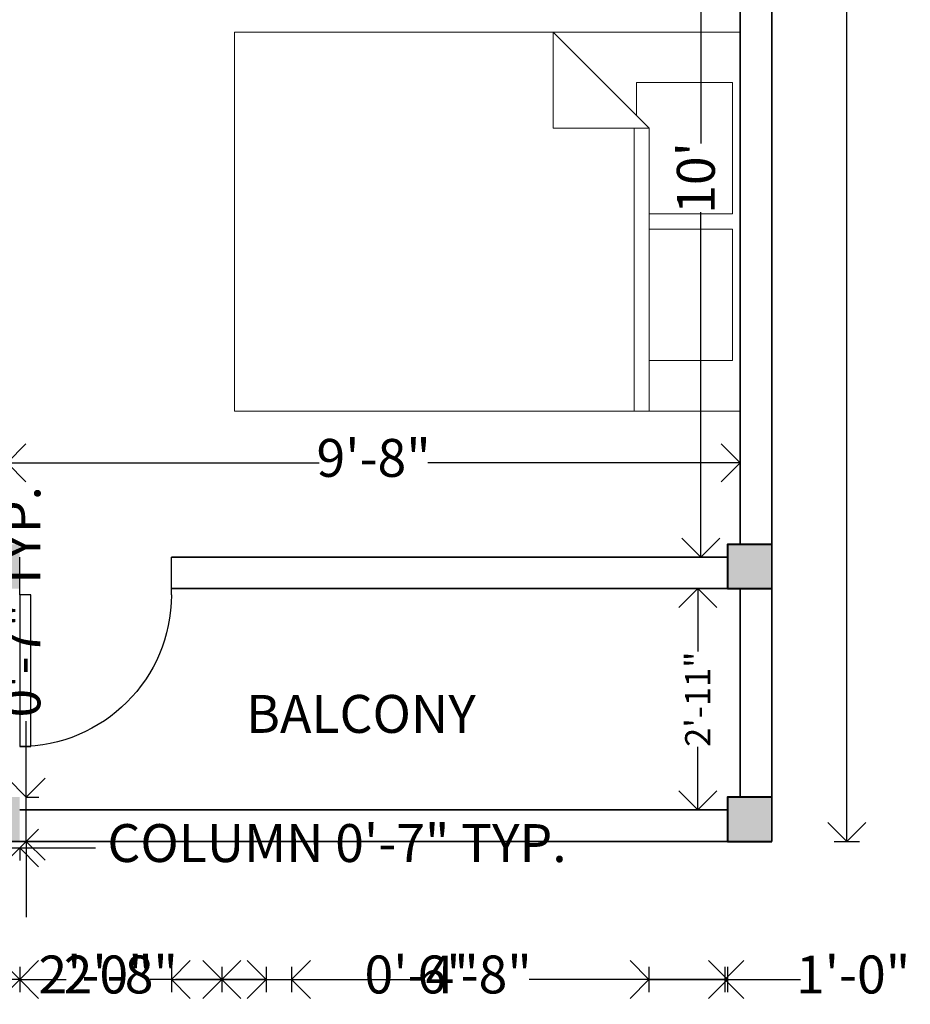
# Model space of a CAD drawing. Units: inches. Extents: x 261 to 714, y 97 to 573.
# Tile 3 of 5: x 541 to 682, y 97 to 253. Entities that reach past the tile are written whole.
import ezdxf

# ---------------------------------------------------------------- set-up
doc = ezdxf.new("R2010")
doc.units = ezdxf.units.IN
for name, color, linetype, lineweight in [('A-ANNO-DIMS', 2, 'Continuous', 18), ('A-AREA-IDEN', 7, 'Continuous', 25), ('A-COLS', 182, 'Continuous', 40), ('A-COLS-PATT', 172, 'Continuous', 13), ('A-DOOR', 182, 'Continuous', 25), ('A-FURN', 8, 'Continuous', 18), ('A-WALL', 182, 'Continuous', 35)]:
    doc.layers.add(name, color=color, linetype=linetype, lineweight=lineweight)
doc.styles.get("Standard").update_dxf_attribs({"font": 'arial.ttf'})
doc.dimstyles.new('ISO-25', dxfattribs={"dimtxt": 6, "dimasz": 6, "dimexe": 2, "dimexo": 2, "dimtad": 0, "dimdec": 1, "dimlunit": 3, "dimtxsty": 'Standard', "dimblk": 'OPEN90', "dimcen": 2.5, "dimclrd": 1, "dimclre": 1, "dimclrt": 1, "dimadec": 0, "dimazin": 0, "dimtfac": 1, "dimtdec": 1, "dimtmove": 0, "dimatfit": 3, "dimfxl": 2, "dimfxlon": 1, "dimarcsym": 0})

# ---------------------------------------------------------------- blocks, each defined once
blk = doc.blocks.new('*U6')
for p, q in [((0, 0), (0, -6)), ((24, 0), (24, -6))]:
    blk.add_line(p, q)
blk.add_lwpolyline([(0, 0), (0, 24), (1.75, 24), (1.75, 0)], close=True)
blk.add_arc((0, 0), 24, 0, 90)
blk = doc.blocks.new('_Open90')
at = {"color": 0, "linetype": 'ByBlock', "lineweight": -2}
for p, q in [((-0.5, 0.5), (0, 0)), ((0, 0), (-1, 0)), ((0, 0), (-0.5, -0.5))]:
    blk.add_line(p, q, dxfattribs=at)
blk = doc.blocks.new('*D21')
at = {"layer": 'A-ANNO-DIMS', "color": 0, "lineweight": -2, "transparency": 16777216}
for p, q in [((646.66, 287.66), (650.66, 287.66)), ((648.66, 281.66), (648.66, 233.09)), ((648.66, 173.66), (648.66, 222.22)), ((646.66, 167.66), (650.66, 167.66))]:
    blk.add_line(p, q, dxfattribs=at)
at = {"layer": 'Defpoints', "color": 0, "transparency": 16777216}
for p in [(643.84, 287.66), (643.84, 167.66), (648.66, 167.66)]:
    blk.add_point(p, dxfattribs=at)
at = {"layer": 'A-ANNO-DIMS', "color": 0, "lineweight": -2, "transparency": 16777216, "xscale": 6, "yscale": 6, "zscale": 6}
for p, rotation in [((648.66, 287.66), 90), ((648.66, 167.66), 270)]:
    blk.add_blockref('_Open90', p, dxfattribs=dict(at, rotation=rotation))
at = {"layer": 'A-ANNO-DIMS', "color": 0, "transparency": 16777216, "insert": (648.66, 227.66), "char_height": 6, "attachment_point": 5, "rotation": 90}
blk.add_mtext("10'", dxfattribs=at)
blk = doc.blocks.new('*D22')
at = {"layer": 'A-ANNO-DIMS', "color": 0, "lineweight": -2, "transparency": 16777216}
for p, q in [((538.9, 184.57), (538.9, 180.57)), ((654.9, 184.57), (654.9, 180.57)), ((544.9, 182.57), (588.3, 182.57)), ((648.9, 182.57), (605.5, 182.57))]:
    blk.add_line(p, q, dxfattribs=at)
at = {"layer": 'Defpoints', "color": 0, "transparency": 16777216}
for p in [(538.9, 189.8), (654.9, 189.8), (654.9, 182.57)]:
    blk.add_point(p, dxfattribs=at)
at = {"layer": 'A-ANNO-DIMS', "color": 0, "lineweight": -2, "transparency": 16777216, "xscale": 6, "yscale": 6, "zscale": 6, "rotation": 180}
blk.add_blockref('_Open90', (538.9, 182.57), dxfattribs=at)
at = {"layer": 'A-ANNO-DIMS', "color": 0, "lineweight": -2, "transparency": 16777216, "xscale": 6, "yscale": 6, "zscale": 6}
blk.add_blockref('_Open90', (654.9, 182.57), dxfattribs=at)
at = {"layer": 'A-ANNO-DIMS', "color": 0, "transparency": 16777216, "insert": (596.9, 182.57), "char_height": 6, "attachment_point": 5}
blk.add_mtext('9\'-8"', dxfattribs=at)
blk = doc.blocks.new('*D24')
at = {"layer": 'A-ANNO-DIMS', "color": 0, "lineweight": -2, "transparency": 16777216}
for p, q in [((650.18, 162.66), (646.18, 162.66)), ((648.18, 156.66), (648.18, 152.69)), ((648.18, 133.66), (648.18, 137.63)), ((650.18, 127.66), (646.18, 127.66))]:
    blk.add_line(p, q, dxfattribs=at)
at = {"layer": 'Defpoints', "color": 0, "transparency": 16777216}
for p in [(662.6, 162.66), (648.18, 127.66), (662.6, 127.66)]:
    blk.add_point(p, dxfattribs=at)
at = {"layer": 'A-ANNO-DIMS', "color": 0, "lineweight": -2, "transparency": 16777216, "xscale": 6, "yscale": 6, "zscale": 6}
for p, rotation in [((648.18, 162.66), 90), ((648.18, 127.66), 270)]:
    blk.add_blockref('_Open90', p, dxfattribs=dict(at, rotation=rotation))
at = {"layer": 'A-ANNO-DIMS', "color": 0, "transparency": 16777216, "insert": (648.18, 145.16), "char_height": 6, "attachment_point": 5, "rotation": 90}
blk.add_mtext('{\\H0.66667x;2\'-11"}', dxfattribs=at)
blk = doc.blocks.new('Bed - Queen')
for p, q in [((0, -80.00003), (0, 0)), ((0, 0), (59.99999, 0)), ((59.99999, 0), (59.99999, -80.00003)), ((7.99999, -1.2), (28.79998, -1.2)), ((7.99999, -14.4), (7.99999, -1.2)), ((28.79998, -1.2), (28.79998, -14.4)), ((31.19999, -1.2), (51.99999, -1.2)), ((31.19999, -14.4), (31.19999, -1.2)), ((51.99999, -1.2), (51.99999, -16.4)), ((0, -14.4), (44.8, -14.4)), ((59.99999, -29.6), (44.8, -14.4)), ((44.8, -14.4), (44.8, -29.6)), ((44.8, -16.8), (0, -16.8)), ((51.99999, -16.4), (46.79936, -16.4)), ((44.8, -29.6), (59.99999, -29.6)), ((59.99999, -80.00003), (0, -80.00003))]:
    blk.add_line(p, q)
blk = doc.blocks.new('*D35')
at = {"layer": 'A-ANNO-DIMS', "color": 0, "lineweight": -2, "transparency": 16777216}
for p, q in [((669.78, 542.66), (673.78, 542.66)), ((671.78, 536.66), (671.78, 338.37)), ((671.78, 128.66), (671.78, 326.94)), ((669.78, 122.66), (673.78, 122.66))]:
    blk.add_line(p, q, dxfattribs=at)
at = {"layer": 'Defpoints', "color": 0, "transparency": 16777216}
for p in [(659.9, 542.66), (659.9, 122.66), (671.78, 122.66)]:
    blk.add_point(p, dxfattribs=at)
at = {"layer": 'A-ANNO-DIMS', "color": 0, "lineweight": -2, "transparency": 16777216, "xscale": 6, "yscale": 6, "zscale": 6}
for p, rotation in [((671.78, 542.66), 90), ((671.78, 122.66), 270)]:
    blk.add_blockref('_Open90', p, dxfattribs=dict(at, rotation=rotation))
at = {"layer": 'A-ANNO-DIMS', "color": 0, "transparency": 16777216, "insert": (671.78, 332.66), "char_height": 6, "attachment_point": 5, "rotation": 90}
blk.add_mtext("35'", dxfattribs=at)
blk = doc.blocks.new('COLUMN-7IN-SIDE-EDGE')
blk.add_lwpolyline([(7, 7), (0, 7), (0, 2), (0, 0), (2, 0), (7, 0)])
blk = doc.blocks.new('*D41')
at = {"layer": 'A-ANNO-DIMS', "color": 1, "lineweight": -2, "transparency": 16777216}
for p, q in [((527.9, 121.61), (521.9, 121.61)), ((533.9, 121.61), (533.9, 119.61)), ((533.9, 121.61), (540.9, 121.61)), ((540.9, 121.61), (540.9, 119.61)), ((546.9, 121.61), (552.9, 121.61))]:
    blk.add_line(p, q, dxfattribs=at)
at = {"layer": 'Defpoints', "color": 0, "transparency": 16777216}
for p in [(533.9, 122.66), (540.9, 122.66), (540.9, 121.61)]:
    blk.add_point(p, dxfattribs=at)
at = {"layer": 'A-ANNO-DIMS', "color": 1, "lineweight": -2, "transparency": 16777216, "xscale": 6, "yscale": 6, "zscale": 6}
blk.add_blockref('_Open90', (533.9, 121.61), dxfattribs=at)
at = {"layer": 'A-ANNO-DIMS', "color": 1, "lineweight": -2, "transparency": 16777216, "xscale": 6, "yscale": 6, "zscale": 6, "rotation": 180}
blk.add_blockref('_Open90', (540.9, 121.61), dxfattribs=at)
at = {"layer": 'A-ANNO-DIMS', "color": 1, "transparency": 16777216, "insert": (591.11, 121.61), "char_height": 6, "attachment_point": 5}
blk.add_mtext('COLUMN 0\'-7" TYP.', dxfattribs=at)
blk = doc.blocks.new('*D42')
at = {"layer": 'A-ANNO-DIMS', "color": 1, "lineweight": -2, "transparency": 16777216}
for p, q in [((541.95, 135.66), (541.95, 141.66)), ((541.95, 129.66), (543.95, 129.66)), ((541.95, 122.66), (541.95, 129.66)), ((541.95, 122.66), (543.95, 122.66)), ((541.95, 116.66), (541.95, 110.66))]:
    blk.add_line(p, q, dxfattribs=at)
at = {"layer": 'Defpoints', "color": 0, "transparency": 16777216}
for p in [(540.9, 129.66), (541.95, 129.66), (540.9, 122.66)]:
    blk.add_point(p, dxfattribs=at)
at = {"layer": 'A-ANNO-DIMS', "color": 1, "lineweight": -2, "transparency": 16777216, "xscale": 6, "yscale": 6, "zscale": 6}
for p, rotation in [((541.95, 129.66), 270), ((541.95, 122.66), 90)]:
    blk.add_blockref('_Open90', p, dxfattribs=dict(at, rotation=rotation))
at = {"layer": 'A-ANNO-DIMS', "color": 1, "transparency": 16777216, "insert": (541.95, 160.57), "char_height": 6, "attachment_point": 5, "rotation": 90}
blk.add_mtext('0\'-7" TYP.', dxfattribs=at)
blk = doc.blocks.new('*D63')
at = {"layer": 'A-ANNO-DIMS', "color": 1, "lineweight": -2, "transparency": 16777216}
for p, q in [((540.9, 102.81), (540.9, 98.81)), ((572.9, 102.81), (572.9, 98.81)), ((546.9, 100.81), (548.25, 100.81)), ((566.9, 100.81), (565.55, 100.81))]:
    blk.add_line(p, q, dxfattribs=at)
at = {"layer": 'Defpoints', "color": 0, "transparency": 16777216}
for p in [(540.9, 287.66), (572.9, 287.66), (572.9, 100.81)]:
    blk.add_point(p, dxfattribs=at)
at = {"layer": 'A-ANNO-DIMS', "color": 1, "lineweight": -2, "transparency": 16777216, "xscale": 6, "yscale": 6, "zscale": 6, "rotation": 180}
blk.add_blockref('_Open90', (540.9, 100.81), dxfattribs=at)
at = {"layer": 'A-ANNO-DIMS', "color": 1, "lineweight": -2, "transparency": 16777216, "xscale": 6, "yscale": 6, "zscale": 6}
blk.add_blockref('_Open90', (572.9, 100.81), dxfattribs=at)
at = {"layer": 'A-ANNO-DIMS', "color": 1, "transparency": 16777216, "insert": (556.9, 100.81), "char_height": 6, "attachment_point": 5}
blk.add_mtext('2\'-8"', dxfattribs=at)
blk = doc.blocks.new('*D64')
at = {"layer": 'A-ANNO-DIMS', "color": 1, "lineweight": -2, "transparency": 16777216}
for p, q in [((572.9, 102.81), (572.9, 98.81)), ((652.88, 102.81), (652.88, 98.81)), ((578.9, 100.81), (604.28, 100.81)), ((646.88, 100.81), (621.51, 100.81))]:
    blk.add_line(p, q, dxfattribs=at)
at = {"layer": 'Defpoints', "color": 0, "transparency": 16777216}
for p in [(572.9, 287.66), (652.88, 287.66), (652.88, 100.81)]:
    blk.add_point(p, dxfattribs=at)
at = {"layer": 'A-ANNO-DIMS', "color": 1, "lineweight": -2, "transparency": 16777216, "xscale": 6, "yscale": 6, "zscale": 6, "rotation": 180}
blk.add_blockref('_Open90', (572.9, 100.81), dxfattribs=at)
at = {"layer": 'A-ANNO-DIMS', "color": 1, "lineweight": -2, "transparency": 16777216, "xscale": 6, "yscale": 6, "zscale": 6}
blk.add_blockref('_Open90', (652.88, 100.81), dxfattribs=at)
at = {"layer": 'A-ANNO-DIMS', "color": 1, "transparency": 16777216, "insert": (612.89, 100.81), "char_height": 6, "attachment_point": 5}
blk.add_mtext('6\'-8"', dxfattribs=at)
blk = doc.blocks.new('*D66')
at = {"layer": 'A-ANNO-DIMS', "color": 1, "lineweight": -2, "transparency": 16777216}
for p, q in [((540.9, 102.81), (540.9, 98.81)), ((564.9, 102.81), (564.9, 98.81)), ((534.9, 100.81), (528.9, 100.81)), ((540.9, 100.81), (544.25, 100.81)), ((564.9, 100.81), (561.55, 100.81)), ((570.9, 100.81), (576.9, 100.81))]:
    blk.add_line(p, q, dxfattribs=at)
at = {"layer": 'Defpoints', "color": 0, "transparency": 16777216}
for p in [(540.9, 162.66), (564.9, 162.66), (564.9, 100.81)]:
    blk.add_point(p, dxfattribs=at)
at = {"layer": 'A-ANNO-DIMS', "color": 1, "lineweight": -2, "transparency": 16777216, "xscale": 6, "yscale": 6, "zscale": 6}
blk.add_blockref('_Open90', (540.9, 100.81), dxfattribs=at)
at = {"layer": 'A-ANNO-DIMS', "color": 1, "lineweight": -2, "transparency": 16777216, "xscale": 6, "yscale": 6, "zscale": 6, "rotation": 180}
blk.add_blockref('_Open90', (564.9, 100.81), dxfattribs=at)
at = {"layer": 'A-ANNO-DIMS', "color": 1, "transparency": 16777216, "insert": (552.9, 100.81), "char_height": 6, "attachment_point": 5}
blk.add_mtext('2\'-0"', dxfattribs=at)
blk = doc.blocks.new('*D69')
at = {"layer": 'A-ANNO-DIMS', "color": 1, "lineweight": -2, "transparency": 16777216}
for p, q in [((579.9, 102.81), (579.9, 98.81)), ((583.9, 102.81), (583.9, 98.81)), ((573.9, 100.81), (567.9, 100.81)), ((579.9, 100.81), (583.9, 100.81)), ((589.9, 100.81), (595.9, 100.81))]:
    blk.add_line(p, q, dxfattribs=at)
at = {"layer": 'Defpoints', "color": 0, "transparency": 16777216}
for p in [(579.9, 328.66), (583.9, 328.66), (583.9, 100.81)]:
    blk.add_point(p, dxfattribs=at)
at = {"layer": 'A-ANNO-DIMS', "color": 1, "lineweight": -2, "transparency": 16777216, "xscale": 6, "yscale": 6, "zscale": 6}
blk.add_blockref('_Open90', (579.9, 100.81), dxfattribs=at)
at = {"layer": 'A-ANNO-DIMS', "color": 1, "lineweight": -2, "transparency": 16777216, "xscale": 6, "yscale": 6, "zscale": 6, "rotation": 180}
blk.add_blockref('_Open90', (583.9, 100.81), dxfattribs=at)
at = {"layer": 'A-ANNO-DIMS', "color": 1, "transparency": 16777216, "insert": (604.5, 100.81), "char_height": 6, "attachment_point": 5}
blk.add_mtext('0\'-4"', dxfattribs=at)
blk = doc.blocks.new('*D75')
at = {"layer": 'A-ANNO-DIMS', "color": 1, "lineweight": -2, "transparency": 16777216}
for p, q in [((640.47, 102.81), (640.47, 98.81)), ((652.46, 102.81), (652.46, 98.81)), ((634.47, 100.81), (628.47, 100.81)), ((640.47, 100.81), (652.46, 100.81)), ((658.46, 100.81), (664.46, 100.81))]:
    blk.add_line(p, q, dxfattribs=at)
at = {"layer": 'Defpoints', "color": 0, "transparency": 16777216}
for p in [(640.47, 328.71), (652.46, 328.71), (652.46, 100.81)]:
    blk.add_point(p, dxfattribs=at)
at = {"layer": 'A-ANNO-DIMS', "color": 1, "lineweight": -2, "transparency": 16777216, "xscale": 6, "yscale": 6, "zscale": 6}
blk.add_blockref('_Open90', (640.47, 100.81), dxfattribs=at)
at = {"layer": 'A-ANNO-DIMS', "color": 1, "lineweight": -2, "transparency": 16777216, "xscale": 6, "yscale": 6, "zscale": 6, "rotation": 180}
blk.add_blockref('_Open90', (652.46, 100.81), dxfattribs=at)
at = {"layer": 'A-ANNO-DIMS', "color": 1, "transparency": 16777216, "insert": (672.77, 100.81), "char_height": 6, "attachment_point": 5}
blk.add_mtext('1\'-0"', dxfattribs=at)

msp = doc.modelspace()

# ---------------------------------------------------------------- hatches: boundary and pattern name
at = {"layer": 'A-COLS-PATT'}
h = msp.add_hatch(color=256, dxfattribs=at)
h.dxf.hatch_style = 1
h.paths.add_polyline_path([(354.9, 542.66), (347.9, 542.66), (347.9, 535.66), (354.9, 535.66)])
h.paths.add_polyline_path([(539.9, 542.66), (532.9, 542.66), (532.9, 537.66), (532.9, 535.66), (534.9, 535.66), (539.9, 535.66), (539.9, 537.66)])
h.paths.add_polyline_path([(474.9, 542.66), (467.9, 542.66), (467.9, 537.66), (467.9, 535.66), (469.9, 535.66), (474.9, 535.66), (474.9, 537.66)])
h.paths.add_polyline_path([(659.9, 542.66), (652.9, 542.66), (652.9, 537.66), (652.9, 535.66), (654.9, 535.66), (659.9, 535.66)])
h.paths.add_polyline_path([(659.9, 395.66), (652.88, 395.66), (652.88, 390.66), (652.88, 388.66), (654.88, 388.66), (659.9, 388.66)])
h.paths.add_polyline_path([(539.9, 395.66), (532.9, 395.66), (532.9, 390.66), (532.9, 388.66), (534.9, 388.66), (539.9, 388.66), (539.9, 390.66)])
h.paths.add_polyline_path([(473.9, 395.66), (466.9, 395.66), (466.9, 394.66), (466.9, 388.66), (473.9, 388.66)])
h.paths.add_polyline_path([(354.9, 394.66), (347.9, 394.66), (347.9, 389.66), (347.9, 387.66), (349.9, 387.66), (354.9, 387.66), (354.9, 389.66)])
h.paths.add_polyline_path([(540.9, 292.66), (533.9, 292.66), (533.9, 287.66), (533.9, 285.66), (535.9, 285.66), (540.9, 285.66), (540.9, 287.66)])
h.paths.add_polyline_path([(659.9, 294.66), (652.88, 294.66), (652.88, 289.66), (652.88, 287.66), (654.88, 287.66), (659.9, 287.66)])
h.paths.add_polyline_path([(473.9, 292.66), (466.9, 292.66), (466.9, 287.66), (466.9, 285.66), (468.9, 285.66), (473.9, 285.66), (473.9, 287.66)])
h.paths.add_polyline_path([(354.9, 293.66), (347.9, 293.66), (347.9, 288.66), (347.9, 286.66), (349.9, 286.66), (354.9, 286.66), (354.9, 288.66)])
h.paths.add_polyline_path([(354.9, 129.66), (347.9, 129.66), (347.9, 124.66), (347.9, 122.66), (349.9, 122.66), (354.9, 122.66), (354.9, 124.66)])
h.paths.add_polyline_path([(354.9, 168.66), (347.9, 168.66), (347.9, 163.66), (347.9, 161.66), (349.9, 161.66), (354.9, 161.66), (354.9, 163.66)])
h.paths.add_polyline_path([(473.9, 169.69), (466.95, 169.69), (466.95, 164.69), (466.95, 162.69), (468.95, 162.69), (473.9, 162.69)])
h.paths.add_polyline_path([(475.9, 129.66), (468.9, 129.66), (468.9, 124.66), (468.9, 122.66), (470.9, 122.66), (475.9, 122.66), (475.9, 124.66)])
h.paths.add_polyline_path([(540.9, 129.66), (533.9, 129.66), (533.9, 124.66), (533.9, 122.66), (535.9, 122.66), (540.9, 122.66), (540.9, 124.66)])
h.paths.add_polyline_path([(540.9, 169.66), (533.9, 169.66), (533.9, 164.66), (533.9, 162.66), (535.9, 162.66), (540.9, 162.66), (540.9, 164.66)])
h.paths.add_polyline_path([(659.9, 169.66), (652.9, 169.66), (652.9, 164.66), (652.9, 162.66), (654.9, 162.66), (659.9, 162.66)])
h.paths.add_polyline_path([(659.9, 129.66), (652.9, 129.66), (652.9, 124.66), (652.9, 122.66), (654.9, 122.66), (659.9, 122.66)])

# ---------------------------------------------------------------- linework, layer by layer
at = {"layer": 'A-WALL'}
for p, q in [((659.9, 122.66), (659.9, 542.66)), ((654.9, 169.66), (654.9, 287.66)), ((564.9, 167.66), (652.9, 167.66)), ((564.9, 162.66), (654.9, 162.66)), ((654.9, 129.66), (654.9, 162.66)), ((540.9, 127.66), (652.9, 127.66)), ((347.9, 122.66), (659.9, 122.66))]:
    msp.add_line(p, q, dxfattribs=at)

# ---------------------------------------------------------------- block references
at = {"layer": 'A-COLS'}
for p in [(652.9, 162.66), (652.9, 122.66)]:
    msp.add_blockref('COLUMN-7IN-SIDE-EDGE', p, dxfattribs=at)
at = {"layer": 'A-DOOR', "xscale": -1, "rotation": 180}
msp.add_blockref('*U6', (540.9, 161.66), dxfattribs=at)
at = {"layer": 'A-FURN', "xscale": -1, "rotation": 270}
msp.add_blockref('Bed - Queen', (654.9, 190.75), dxfattribs=at)

# ---------------------------------------------------------------- texts
at = {"layer": 'A-AREA-IDEN', "insert": (576.71, 145.83), "char_height": 6, "attachment_point": 1}
msp.add_mtext_dynamic_manual_height_columns('{BALCONY}', width=60.8654, gutter_width=12.5, heights=[0], dxfattribs=at)

# ---------------------------------------------------------------- dimensions: what is measured, and where the dimension line sits
at = {"layer": 'A-ANNO-DIMS'}
for base, p1, p2, picture, middle in [((671.78, 122.66), (659.9, 542.66), (659.9, 122.66), '*D35', (671.78, 332.66)), ((648.66, 167.66), (643.84, 287.66), (643.84, 167.66), '*D21', (648.66, 227.66))]:
    dim = msp.add_linear_dim(base=base, p1=p1, p2=p2, angle=90, dimstyle='ISO-25', override={"dimclrd": 0, "dimclre": 0, "dimclrt": 0}, dxfattribs=at)
    dim.commit()
    dim.dimension.update_dxf_attribs({"geometry": picture, "text_midpoint": middle})
for base, p1, p2, picture, middle in [((583.9, 100.81), (579.9, 328.66), (583.9, 328.66), '*D69', (604.5, 100.81)), ((652.46, 100.81), (640.47, 328.71), (652.46, 328.71), '*D75', (672.77, 100.81)), ((572.9, 100.81), (540.9, 287.66), (572.9, 287.66), '*D63', (556.9, 100.81)), ((652.88, 100.81), (572.9, 287.66), (652.88, 287.66), '*D64', (612.89, 100.81)), ((564.9, 100.81), (540.9, 162.66), (564.9, 162.66), '*D66', (552.9, 100.81))]:
    dim = msp.add_linear_dim(base=base, p1=p1, p2=p2, dimstyle='ISO-25', override={"dimdec": 1, "dimlfac": 1, "dimrnd": 0, "dimzin": 1, "dimdsep": 46, "dimlunit": 4, "dimfrac": 2}, dxfattribs=at)
    dim.commit()
    dim.dimension.update_dxf_attribs({"geometry": picture, "text_midpoint": middle})
dim = msp.add_linear_dim(base=(654.9, 182.57), p1=(538.9, 189.8), p2=(654.9, 189.8), dimstyle='ISO-25', override={"dimclrd": 0, "dimclre": 0, "dimclrt": 0}, dxfattribs=at)
dim.commit()
dim.dimension.update_dxf_attribs({"geometry": '*D22', "text_midpoint": (596.9, 182.57), "dimtype": 160})
for base, p1, p2, text, override, picture, middle in [((541.95, 129.66), (540.9, 122.66), (540.9, 129.66), '<> TYP.', {"dimdec": 1, "dimlfac": 1, "dimrnd": 0, "dimzin": 1, "dimdsep": 46, "dimlunit": 4, "dimfrac": 2}, '*D42', (541.95, 160.57)), ((648.18, 127.66), (662.6, 162.66), (662.6, 127.66), '{\\H0.66667x;<>}', {"dimclrd": 0, "dimclre": 0, "dimclrt": 0}, '*D24', (648.18, 145.16))]:
    dim = msp.add_linear_dim(base=base, p1=p1, p2=p2, angle=90, text=text, dimstyle='ISO-25', override=override, dxfattribs=at)
    dim.commit()
    dim.dimension.update_dxf_attribs({"geometry": picture, "text_midpoint": middle})
dim = msp.add_linear_dim(base=(540.9, 121.61), p1=(533.9, 122.66), p2=(540.9, 122.66), text='COLUMN <> TYP.', dimstyle='ISO-25', override={"dimdec": 1, "dimlfac": 1, "dimrnd": 0, "dimzin": 1, "dimdsep": 46, "dimlunit": 4, "dimfrac": 2}, dxfattribs=at)
dim.commit()
dim.dimension.update_dxf_attribs({"geometry": '*D41', "text_midpoint": (591.11, 121.61)})

doc.saveas('drawing.dxf')
